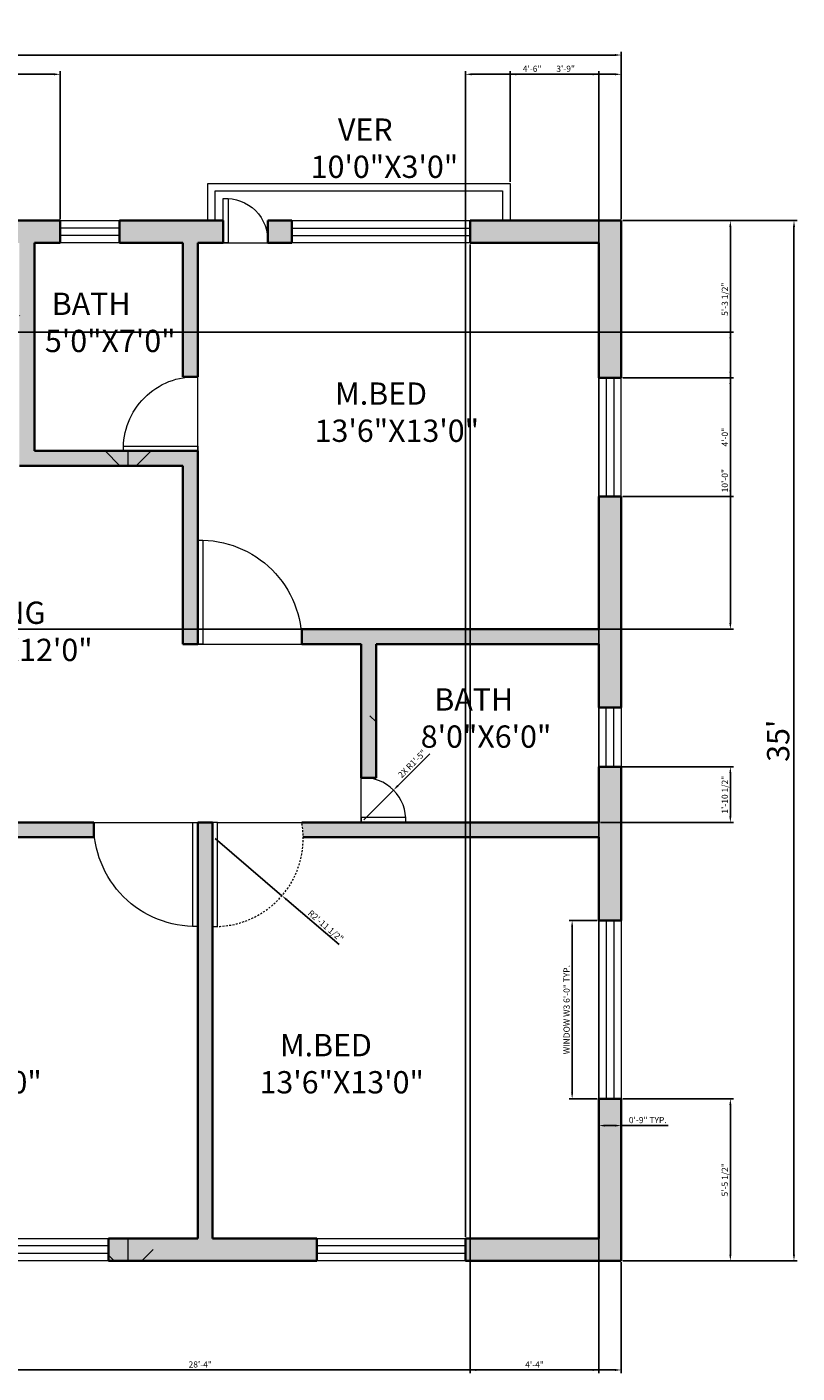
# Model space of a CAD drawing. Units: inches. Extents: x 1851 to 3979, y 3948 to 8145.
# Tile 4 of 4: x 2438 to 2749, y 3948 to 4491. Entities that reach past the tile are written whole.
import ezdxf

# ---------------------------------------------------------------- set-up
doc = ezdxf.new("R2010")
doc.units = ezdxf.units.IN
doc.linetypes.add('JIS_02_0.7', pattern=[1.35, 0.75, -0.6])
for name, color, linetype, lineweight in [('A-ANNO-DIMS', 2, 'Continuous', 18), ('A-GLAZ', 140, 'Continuous', 18), ('A-WALL', 7, 'Continuous', 35)]:
    doc.layers.add(name, color=color, linetype=linetype, lineweight=lineweight)
for name, color, linetype, lineweight, true_color in [('A-AREA-IDEN', 9, 'Continuous', 18, 0xc7c8ca), ('A-DOOR', 52, 'Continuous', 18, 0xc8c92d), ('A-DOOR-SWNG', 52, 'JIS_02_0.7', 13, 0xc8c92d), ('A-FLOR-RAIL', 52, 'Continuous', 18, 0xc8c92d), ('A-WALL-PATT', 159, 'Continuous', 13, 0x22346e)]:
    doc.layers.add(name, color=color, linetype=linetype, lineweight=lineweight, true_color=true_color)
doc.styles.get("Standard").update_dxf_attribs({"font": 'arial.ttf'})
doc.dimstyles.new('ISO-25', dxfattribs={"dimtxt": 2.5, "dimasz": 2.5, "dimexe": 1.25, "dimexo": 0.625, "dimtad": 1, "dimlunit": 3, "dimtxsty": 'Standard', "dimcen": 2.5, "dimadec": 0, "dimazin": 0, "dimtfac": 1, "dimtmove": 0, "dimatfit": 3, "dimfxl": 1, "dimarcsym": 0})

# ---------------------------------------------------------------- blocks, each defined once
blk = doc.blocks.new('*D1')
at = {"layer": 'A-ANNO-DIMS', "color": 0, "lineweight": -2, "transparency": 16777216}
for p, q in [((1898.74, 4438.02), (1898.74, 4480.98)), ((1901.24, 4479.73), (2675.24, 4479.73)), ((2677.74, 4438.02), (2677.74, 4480.98))]:
    blk.add_line(p, q, dxfattribs=at)
at = {"layer": 'A-ANNO-DIMS', "color": 0, "transparency": 16777216}
for points in [[(1901.24, 4480.15), (1901.24, 4479.31), (1898.74, 4479.73)], [(2675.24, 4480.15), (2675.24, 4479.31), (2677.74, 4479.73)]]:
    blk.add_solid(points, dxfattribs=at)
at = {"layer": 'Defpoints', "color": 0, "transparency": 16777216}
for p in [(2677.74, 4479.73), (1898.74, 4437.39), (2677.74, 4437.39)]:
    blk.add_point(p, dxfattribs=at)
at = {"layer": 'A-ANNO-DIMS', "color": 0, "transparency": 16777216, "insert": (2288.24, 4484.95), "char_height": 9, "attachment_point": 5}
blk.add_mtext('64\'-11"', dxfattribs=at)
blk = doc.blocks.new('*D2')
at = {"layer": 'A-ANNO-DIMS', "color": 0, "lineweight": -2, "transparency": 16777216}
for p, q in [((2712.32, 4412.85), (2748.78, 4412.85)), ((2747.53, 4410.35), (2747.53, 3995.35)), ((2699.58, 3992.85), (2748.78, 3992.85))]:
    blk.add_line(p, q, dxfattribs=at)
at = {"layer": 'A-ANNO-DIMS', "color": 0, "transparency": 16777216}
for points in [[(2747.12, 4410.35), (2747.95, 4410.35), (2747.53, 4412.85)], [(2747.12, 3995.35), (2747.95, 3995.35), (2747.53, 3992.85)]]:
    blk.add_solid(points, dxfattribs=at)
at = {"layer": 'Defpoints', "color": 0, "transparency": 16777216}
for p in [(2711.7, 4412.85), (2698.96, 3992.85), (2747.53, 3992.85)]:
    blk.add_point(p, dxfattribs=at)
at = {"layer": 'A-ANNO-DIMS', "color": 0, "transparency": 16777216, "insert": (2742.31, 4202.85), "char_height": 9, "attachment_point": 5, "rotation": 90}
blk.add_mtext("35'", dxfattribs=at)
blk = doc.blocks.new('DOOR-SINGLE-42IN')
for p, q in [((42, 42), (40, 42)), ((40, 42), (40, 0)), ((42, 0), (42, 42)), ((40, 0), (42, 0))]:
    blk.add_line(p, q)
blk.add_arc((41, 1), 41.01, 88.6028, 181.3972)
blk = doc.blocks.new('DOOR-SINGLE-30IN')
for p, q in [((30, 2), (0, 2)), ((0, 2), (0, 0)), ((0, 0), (30, 0)), ((30, 0), (30, 2))]:
    blk.add_line(p, q)
blk.add_arc((1, 1), 29.02, 358.0251, 91.9749)
blk = doc.blocks.new('DOOR-SINGLE-18IN')
for p, q in [((18, 18), (16, 18)), ((16, 18), (16, 0)), ((18, 0), (18, 18)), ((16, 0), (18, 0))]:
    blk.add_line(p, q)
blk.add_arc((17, 1), 17.03, 86.6335, 183.3665)
blk = doc.blocks.new('WINDOW-60IN')
for p, q in [((0, 9), (60, 9)), ((0, 0), (0, 9)), ((0, 6), (60, 6)), ((60, 9), (60, 0)), ((0, 3), (60, 3)), ((60, 0), (0, 0))]:
    blk.add_line(p, q)
blk = doc.blocks.new('WINDOW-24IN')
for p, q in [((0, 0), (0, 9)), ((0, 9), (24, 9)), ((0, 6), (24, 6)), ((24, 9), (24, 0)), ((0, 3), (24, 3)), ((24, 0), (0, 0))]:
    blk.add_line(p, q)
blk = doc.blocks.new('WINDOW-72IN')
for p, q in [((0, 9), (72, 9)), ((0, 0), (0, 9)), ((0, 6), (72, 6)), ((72, 9), (72, 0)), ((0, 3), (72, 3)), ((72, 0), (0, 0))]:
    blk.add_line(p, q)
blk = doc.blocks.new('*D14')
at = {"layer": 'A-ANNO-DIMS', "color": 0, "lineweight": -2, "transparency": 16777216}
for p, q in [((2668.11, 4130.25), (2656.69, 4130.25)), ((2657.94, 4127.75), (2657.94, 4060.75)), ((2668.11, 4058.25), (2656.69, 4058.25))]:
    blk.add_line(p, q, dxfattribs=at)
at = {"layer": 'A-ANNO-DIMS', "color": 0, "transparency": 16777216}
for points in [[(2657.52, 4127.75), (2658.35, 4127.75), (2657.94, 4130.25)], [(2657.52, 4060.75), (2658.35, 4060.75), (2657.94, 4058.25)]]:
    blk.add_solid(points, dxfattribs=at)
at = {"layer": 'Defpoints', "color": 0, "transparency": 16777216}
for p in [(2668.74, 4130.25), (2657.94, 4058.25), (2668.74, 4058.25)]:
    blk.add_point(p, dxfattribs=at)
at = {"layer": 'A-ANNO-DIMS', "color": 0, "transparency": 16777216, "insert": (2656.02, 4094.25), "char_height": 2.5, "attachment_point": 5, "rotation": 90}
blk.add_mtext('WINDOW W3 6\'-0" TYP.', dxfattribs=at)
blk = doc.blocks.new('*D15')
at = {"layer": 'A-ANNO-DIMS', "color": 0, "lineweight": -2, "transparency": 16777216}
for p, q in [((2668.74, 4057.63), (2668.74, 4046.2)), ((2677.74, 4057.63), (2677.74, 4046.2)), ((2671.24, 4047.45), (2675.24, 4047.45)), ((2677.74, 4047.45), (2696.72, 4047.45))]:
    blk.add_line(p, q, dxfattribs=at)
at = {"layer": 'A-ANNO-DIMS', "color": 0, "transparency": 16777216}
for points in [[(2671.24, 4047.87), (2671.24, 4047.03), (2668.74, 4047.45)], [(2675.24, 4047.87), (2675.24, 4047.03), (2677.74, 4047.45)]]:
    blk.add_solid(points, dxfattribs=at)
at = {"layer": 'Defpoints', "color": 0, "transparency": 16777216}
for p in [(2668.74, 4058.25), (2677.74, 4058.25), (2677.74, 4047.45)]:
    blk.add_point(p, dxfattribs=at)
at = {"layer": 'A-ANNO-DIMS', "color": 0, "transparency": 16777216, "insert": (2688.48, 4049.35), "char_height": 2.5, "attachment_point": 5}
blk.add_mtext('0\'-9" TYP.', dxfattribs=at)
blk = doc.blocks.new('*D26')
at = {"layer": 'A-ANNO-DIMS', "color": 0, "lineweight": -2, "transparency": 16777216}
for p, q in [((2337.74, 3992.23), (2337.74, 3947.5)), ((2677.74, 3992.23), (2677.74, 3947.5)), ((2340.24, 3948.75), (2675.24, 3948.75))]:
    blk.add_line(p, q, dxfattribs=at)
at = {"layer": 'A-ANNO-DIMS', "color": 0, "transparency": 16777216}
for points in [[(2340.24, 3949.17), (2340.24, 3948.34), (2337.74, 3948.75)], [(2675.24, 3949.17), (2675.24, 3948.34), (2677.74, 3948.75)]]:
    blk.add_solid(points, dxfattribs=at)
at = {"layer": 'Defpoints', "color": 0, "transparency": 16777216}
for p in [(2337.74, 3992.85), (2677.74, 3992.85), (2677.74, 3948.75)]:
    blk.add_point(p, dxfattribs=at)
at = {"layer": 'A-ANNO-DIMS', "color": 0, "transparency": 16777216, "insert": (2507.74, 3950.66), "char_height": 2.5, "attachment_point": 5}
blk.add_mtext('28\'-4"', dxfattribs=at)
blk = doc.blocks.new('*D30')
at = {"layer": 'A-ANNO-DIMS', "color": 0, "lineweight": -2, "transparency": 16777216}
for p, q in [((2614.83, 4002.48), (2614.83, 4473.2)), ((2617.33, 4471.95), (2666.24, 4471.95)), ((2668.74, 4002.48), (2668.74, 4473.2))]:
    blk.add_line(p, q, dxfattribs=at)
at = {"layer": 'A-ANNO-DIMS', "color": 0, "transparency": 16777216}
for points in [[(2617.33, 4472.37), (2617.33, 4471.54), (2614.83, 4471.95)], [(2666.24, 4472.37), (2666.24, 4471.54), (2668.74, 4471.95)]]:
    blk.add_solid(points, dxfattribs=at)
at = {"layer": 'Defpoints', "color": 0, "transparency": 16777216}
for p in [(2668.74, 4471.95), (2614.83, 4001.85), (2668.74, 4001.85)]:
    blk.add_point(p, dxfattribs=at)
at = {"layer": 'A-ANNO-DIMS', "color": 0, "transparency": 16777216, "insert": (2641.78, 4473.86), "char_height": 2.5, "attachment_point": 5}
blk.add_mtext('4\'-6"', dxfattribs=at)
blk = doc.blocks.new('*D32')
at = {"layer": 'A-ANNO-DIMS', "color": 0, "lineweight": -2, "transparency": 16777216}
for p, q in [((2632.88, 4428.48), (2632.88, 4473.2)), ((2635.38, 4471.95), (2675.24, 4471.95)), ((2677.74, 4413.48), (2677.74, 4473.2))]:
    blk.add_line(p, q, dxfattribs=at)
at = {"layer": 'A-ANNO-DIMS', "color": 0, "transparency": 16777216}
for points in [[(2635.38, 4472.37), (2635.38, 4471.54), (2632.88, 4471.95)], [(2675.24, 4472.37), (2675.24, 4471.54), (2677.74, 4471.95)]]:
    blk.add_solid(points, dxfattribs=at)
at = {"layer": 'Defpoints', "color": 0, "transparency": 16777216}
for p in [(2677.74, 4471.95), (2632.88, 4427.85), (2677.74, 4412.85)]:
    blk.add_point(p, dxfattribs=at)
at = {"layer": 'A-ANNO-DIMS', "color": 0, "transparency": 16777216, "insert": (2655.31, 4473.86), "char_height": 2.5, "attachment_point": 5}
blk.add_mtext('3\'-9"', dxfattribs=at)
blk = doc.blocks.new('*D33')
at = {"layer": 'A-ANNO-DIMS', "color": 0, "lineweight": -2, "transparency": 16777216}
for p, q in [((2245.36, 4367.85), (2723.09, 4367.85)), ((2721.84, 4250.35), (2721.84, 4365.35)), ((2245.36, 4247.85), (2723.09, 4247.85))]:
    blk.add_line(p, q, dxfattribs=at)
at = {"layer": 'A-ANNO-DIMS', "color": 0, "transparency": 16777216}
for points in [[(2721.42, 4365.35), (2722.25, 4365.35), (2721.84, 4367.85)], [(2721.42, 4250.35), (2722.25, 4250.35), (2721.84, 4247.85)]]:
    blk.add_solid(points, dxfattribs=at)
at = {"layer": 'Defpoints', "color": 0, "transparency": 16777216}
for p in [(2244.74, 4367.85), (2721.84, 4367.85), (2244.74, 4247.85)]:
    blk.add_point(p, dxfattribs=at)
at = {"layer": 'A-ANNO-DIMS', "color": 0, "transparency": 16777216, "insert": (2719.93, 4307.85), "char_height": 2.5, "attachment_point": 5, "rotation": 90}
blk.add_mtext('10\'-0"', dxfattribs=at)
blk = doc.blocks.new('*D40')
at = {"layer": 'A-ANNO-DIMS', "color": 0, "lineweight": -2, "transparency": 16777216}
for p, q in [((2678.36, 4058.25), (2723.09, 4058.25)), ((2721.84, 3995.35), (2721.84, 4055.75)), ((2678.36, 3992.85), (2723.09, 3992.85))]:
    blk.add_line(p, q, dxfattribs=at)
at = {"layer": 'A-ANNO-DIMS', "color": 0, "transparency": 16777216}
for points in [[(2721.42, 4055.75), (2722.25, 4055.75), (2721.84, 4058.25)], [(2721.42, 3995.35), (2722.25, 3995.35), (2721.84, 3992.85)]]:
    blk.add_solid(points, dxfattribs=at)
at = {"layer": 'Defpoints', "color": 0, "transparency": 16777216}
for p in [(2677.74, 4058.25), (2721.84, 4058.25), (2677.74, 3992.85)]:
    blk.add_point(p, dxfattribs=at)
at = {"layer": 'A-ANNO-DIMS', "color": 0, "transparency": 16777216, "insert": (2719.92, 4025.55), "char_height": 2.5, "attachment_point": 5, "rotation": 90}
blk.add_mtext('5\'-5 1/2"', dxfattribs=at)
blk = doc.blocks.new('*D41')
at = {"layer": 'A-ANNO-DIMS', "color": 0, "lineweight": -2, "transparency": 16777216}
for p, q in [((2669.36, 4192.25), (2723.09, 4192.25)), ((2721.84, 4172.35), (2721.84, 4189.75)), ((2669.36, 4169.85), (2723.09, 4169.85))]:
    blk.add_line(p, q, dxfattribs=at)
at = {"layer": 'A-ANNO-DIMS', "color": 0, "transparency": 16777216}
for points in [[(2721.42, 4189.75), (2722.25, 4189.75), (2721.84, 4192.25)], [(2721.42, 4172.35), (2722.25, 4172.35), (2721.84, 4169.85)]]:
    blk.add_solid(points, dxfattribs=at)
at = {"layer": 'Defpoints', "color": 0, "transparency": 16777216}
for p in [(2668.74, 4192.25), (2721.84, 4192.25), (2668.74, 4169.85)]:
    blk.add_point(p, dxfattribs=at)
at = {"layer": 'A-ANNO-DIMS', "color": 0, "transparency": 16777216, "insert": (2719.92, 4181.05), "char_height": 2.5, "attachment_point": 5, "rotation": 90}
blk.add_mtext('1\'-10 1/2"', dxfattribs=at)
blk = doc.blocks.new('*D42')
at = {"layer": 'A-ANNO-DIMS', "color": 0, "lineweight": -2, "transparency": 16777216}
for p, q in [((2678.36, 4349.41), (2723.09, 4349.41)), ((2721.84, 4303.91), (2721.84, 4346.91)), ((2678.36, 4301.41), (2723.09, 4301.41))]:
    blk.add_line(p, q, dxfattribs=at)
at = {"layer": 'A-ANNO-DIMS', "color": 0, "transparency": 16777216}
for points in [[(2721.42, 4346.91), (2722.25, 4346.91), (2721.84, 4349.41)], [(2721.42, 4303.91), (2722.25, 4303.91), (2721.84, 4301.41)]]:
    blk.add_solid(points, dxfattribs=at)
at = {"layer": 'Defpoints', "color": 0, "transparency": 16777216}
for p in [(2677.74, 4349.41), (2721.84, 4349.41), (2677.74, 4301.41)]:
    blk.add_point(p, dxfattribs=at)
at = {"layer": 'A-ANNO-DIMS', "color": 0, "transparency": 16777216, "insert": (2719.93, 4325.41), "char_height": 2.5, "attachment_point": 5, "rotation": 90}
blk.add_mtext('4\'-0"', dxfattribs=at)
blk = doc.blocks.new('*D43')
at = {"layer": 'A-ANNO-DIMS', "color": 0, "lineweight": -2, "transparency": 16777216}
for p, q in [((2678.36, 4412.85), (2723.09, 4412.85)), ((2721.84, 4351.91), (2721.84, 4410.35)), ((2678.36, 4349.41), (2723.09, 4349.41))]:
    blk.add_line(p, q, dxfattribs=at)
at = {"layer": 'A-ANNO-DIMS', "color": 0, "transparency": 16777216}
for points in [[(2721.42, 4410.35), (2722.25, 4410.35), (2721.84, 4412.85)], [(2721.42, 4351.91), (2722.25, 4351.91), (2721.84, 4349.41)]]:
    blk.add_solid(points, dxfattribs=at)
at = {"layer": 'Defpoints', "color": 0, "transparency": 16777216}
for p in [(2677.74, 4412.85), (2721.84, 4412.85), (2677.74, 4349.41)]:
    blk.add_point(p, dxfattribs=at)
at = {"layer": 'A-ANNO-DIMS', "color": 0, "transparency": 16777216, "insert": (2719.92, 4381.13), "char_height": 2.5, "attachment_point": 5, "rotation": 90}
blk.add_mtext('5\'-3 1/2"', dxfattribs=at)
blk = doc.blocks.new('*D47')
at = {"layer": 'A-ANNO-DIMS', "color": 0, "lineweight": -2, "transparency": 16777216}
for p, q in [((2616.74, 4403.23), (2616.74, 3947.5)), ((2668.74, 4403.23), (2668.74, 3947.5)), ((2619.24, 3948.75), (2666.24, 3948.75))]:
    blk.add_line(p, q, dxfattribs=at)
at = {"layer": 'A-ANNO-DIMS', "color": 0, "transparency": 16777216}
for points in [[(2619.24, 3949.17), (2619.24, 3948.34), (2616.74, 3948.75)], [(2666.24, 3949.17), (2666.24, 3948.34), (2668.74, 3948.75)]]:
    blk.add_solid(points, dxfattribs=at)
at = {"layer": 'Defpoints', "color": 0, "transparency": 16777216}
for p in [(2616.74, 4403.85), (2668.74, 4403.85), (2668.74, 3948.75)]:
    blk.add_point(p, dxfattribs=at)
at = {"layer": 'A-ANNO-DIMS', "color": 0, "transparency": 16777216, "insert": (2642.74, 3950.63), "char_height": 2.5, "attachment_point": 5}
blk.add_mtext('4\'-4"', dxfattribs=at)
blk = doc.blocks.new('*D52')
at = {"layer": 'A-ANNO-DIMS', "color": 0, "lineweight": -2, "transparency": 16777216}
for p, q in [((2401.88, 4413.48), (2401.88, 4473.2)), ((2404.38, 4471.95), (2448.67, 4471.95)), ((2451.17, 4413.48), (2451.17, 4473.2))]:
    blk.add_line(p, q, dxfattribs=at)
at = {"layer": 'A-ANNO-DIMS', "color": 0, "transparency": 16777216}
for points in [[(2404.38, 4472.37), (2404.38, 4471.54), (2401.88, 4471.95)], [(2448.67, 4472.37), (2448.67, 4471.54), (2451.17, 4471.95)]]:
    blk.add_solid(points, dxfattribs=at)
at = {"layer": 'Defpoints', "color": 0, "transparency": 16777216}
for p in [(2451.17, 4471.95), (2401.88, 4412.85), (2451.17, 4412.85)]:
    blk.add_point(p, dxfattribs=at)
at = {"layer": 'A-ANNO-DIMS', "color": 0, "transparency": 16777216, "insert": (2426.53, 4473.87), "char_height": 2.5, "attachment_point": 5}
blk.add_mtext('4\'-1 1/2"', dxfattribs=at)
blk = doc.blocks.new('*D54')
at = {"layer": 'A-ANNO-DIMS', "color": 0, "lineweight": -2, "transparency": 16777216}
for p, q in [((2513.74, 4163.43), (2540.75, 4140.27)), ((2563.82, 4120.5), (2542.65, 4138.64))]:
    blk.add_line(p, q, dxfattribs=at)
at = {"layer": 'A-ANNO-DIMS', "color": 0, "transparency": 16777216}
blk.add_solid([(2542.92, 4138.96), (2542.38, 4138.32), (2540.75, 4140.27)], dxfattribs=at)
at = {"layer": 'Defpoints', "color": 0, "transparency": 16777216}
for p in [(2513.74, 4163.43), (2540.75, 4140.27)]:
    blk.add_point(p, dxfattribs=at)
at = {"layer": 'A-ANNO-DIMS', "color": 0, "transparency": 16777216, "insert": (2558.21, 4127.83), "char_height": 2.5, "attachment_point": 5, "rotation": 319.3996}
blk.add_mtext('R2\'-11 1/2"', dxfattribs=at)
blk = doc.blocks.new('*D56')
at = {"layer": 'A-ANNO-DIMS', "color": 0, "lineweight": -2, "transparency": 16777216}
for p, q in [((2600.42, 4197.54), (2587.55, 4184.66)), ((2573.74, 4170.85), (2585.78, 4182.9))]:
    blk.add_line(p, q, dxfattribs=at)
at = {"layer": 'A-ANNO-DIMS', "color": 0, "transparency": 16777216}
blk.add_solid([(2587.25, 4184.96), (2587.84, 4184.37), (2585.78, 4182.9)], dxfattribs=at)
at = {"layer": 'Defpoints', "color": 0, "transparency": 16777216}
for p in [(2585.78, 4182.9), (2573.74, 4170.85)]:
    blk.add_point(p, dxfattribs=at)
at = {"layer": 'A-ANNO-DIMS', "color": 0, "transparency": 16777216, "insert": (2593.52, 4193.33), "char_height": 2.5, "attachment_point": 5, "rotation": 45.0002}
blk.add_mtext('2X R1\'-5"', dxfattribs=at)

msp = doc.modelspace()

# ---------------------------------------------------------------- hatches: boundary and pattern name
at = {"layer": 'A-WALL-PATT'}
h = msp.add_hatch(dxfattribs=at)
h.set_pattern_fill('GRASS', color=256, scale=3)
h.paths.add_polyline_path([(1942.655, 4412.855), (1898.736, 4412.855), (1898.736, 4348.625), (1907.736, 4348.625), (1907.736, 4403.855), (1942.655, 4403.855)])
h.paths.add_polyline_path([(2027.97, 4412.855), (2002.655, 4412.855), (2002.655, 4403.855), (2027.97, 4403.855, -0.0293864), (2027.97, 4405.855)])
h.paths.add_polyline_path([(2088.59, 4412.855), (2045.97, 4412.855), (2045.97, 4403.855), (2069.736, 4403.855), (2069.736, 4349.855, -0.0172363), (2071.736, 4349.855), (2075.736, 4349.855), (2075.736, 4403.855), (2088.59, 4403.855)])
h.paths.add_polyline_path([(2158.724, 4412.855), (2112.59, 4412.855), (2112.59, 4403.855), (2135.736, 4403.855), (2135.736, 4319.855), (2069.736, 4319.855), (2069.736, 4241.855), (2075.736, 4241.855), (2075.736, 4313.855), (2141.736, 4313.855), (2141.736, 4403.855), (2158.724, 4403.855)])
h.paths.add_polyline_path([(2244.736, 4403.855), (2256.687, 4403.855), (2256.687, 4412.855), (2218.724, 4412.855), (2218.724, 4403.855), (2238.736, 4403.855), (2238.736, 4319.855), (2171.736, 4319.855), (2171.736, 4315.855, -0.0172363), (2171.736, 4313.855), (2238.736, 4313.855), (2238.736, 4211.855), (2242.736, 4211.855, -0.0121933), (2244.736, 4211.855)])
h.paths.add_polyline_path([(2356.912, 4412.855), (2353.884, 4412.855), (2312.372, 4412.855), (2312.372, 4403.855), (2331.736, 4403.855), (2331.736, 4211.855, -0.0121933), (2333.736, 4211.855), (2337.736, 4211.855), (2337.736, 4313.855), (2404.736, 4313.855, -0.0172363), (2404.736, 4315.855), (2404.736, 4319.855), (2337.736, 4319.855), (2337.736, 4403.855), (2353.884, 4403.855), (2356.912, 4403.855)])
h.paths.add_polyline_path([(2440.736, 4403.855), (2451.168, 4403.855), (2451.168, 4412.855), (2401.884, 4412.855), (2401.884, 4403.855), (2434.736, 4403.855), (2434.736, 4313.855), (2500.736, 4313.855), (2500.736, 4241.855), (2506.736, 4241.855), (2506.736, 4283.855), (2506.736, 4319.855), (2476.736, 4319.855), (2440.736, 4319.855)])
h.paths.add_polyline_path([(2506.736, 4403.855), (2516.983, 4403.855), (2516.983, 4412.855), (2475.168, 4412.855), (2475.168, 4403.855), (2500.736, 4403.855), (2500.736, 4349.855), (2504.736, 4349.855, -0.0172363), (2506.736, 4349.855)])
h.paths.add_polyline_path([(2544.739, 4412.855), (2534.983, 4412.855), (2534.983, 4405.855, -0.0293864), (2534.983, 4403.855), (2544.739, 4403.855)])
h.paths.add_polyline_path([(2677.736, 4412.855), (2618.736, 4412.855), (2616.739, 4412.855), (2616.739, 4403.855), (2668.736, 4403.855), (2668.736, 4349.414), (2677.736, 4349.414), (2677.736, 4403.855)])
h.paths.add_polyline_path([(2677.736, 4301.414), (2668.736, 4301.414), (2668.736, 4247.855), (2548.736, 4247.855), (2548.736, 4243.855, -0.0121933), (2548.736, 4241.855), (2572.736, 4241.855), (2572.736, 4187.855, -0.0293864), (2574.736, 4187.855), (2578.736, 4187.855), (2578.736, 4241.855), (2668.736, 4241.855), (2668.736, 4216.247), (2677.736, 4216.247)])
h.paths.add_polyline_path([(2677.736, 4192.247), (2668.736, 4192.247), (2668.736, 4169.855), (2572.736, 4169.855), (2548.736, 4169.855, -0.0424267), (2549.319, 4163.855), (2572.736, 4163.855), (2668.736, 4163.855), (2668.736, 4130.251), (2677.736, 4130.251)])
h.paths.add_polyline_path([(2677.736, 4001.855), (2677.736, 4058.251), (2668.736, 4058.251), (2668.736, 4001.855), (2614.828, 4001.855), (2614.828, 3992.855), (2618.736, 3992.855), (2677.736, 3992.855)])
h.paths.add_polyline_path([(2554.828, 4001.855), (2512.736, 4001.855), (2512.736, 4163.855), (2512.736, 4169.855), (2506.736, 4169.855), (2506.736, 4127.855), (2506.736, 4001.855), (2470.736, 4001.855), (2470.736, 3992.855), (2554.828, 3992.855)])
h.paths.add_polyline_path([(2410.736, 4001.855), (2337.736, 4001.855), (2337.736, 3992.855), (2410.736, 3992.855)])
h.paths.add_polyline_path([(2337.736, 4169.855), (2331.736, 4169.855), (2331.736, 4075.855), (2337.736, 4075.855)])
h.paths.add_polyline_path([(2464.736, 4167.855, -0.0121933), (2464.736, 4169.855), (2337.736, 4169.855), (2337.736, 4163.855), (2464.736, 4163.855)])
h.paths.add_polyline_path([(2244.736, 4169.855), (2202.736, 4169.855), (2117.736, 4169.855, -0.0121933), (2117.736, 4167.855), (2117.736, 4163.855), (2238.736, 4163.855), (2238.736, 4075.855), (2244.736, 4075.855)])
h.paths.add_polyline_path([(2325.736, 4001.855), (2250.736, 4001.855), (2250.736, 3992.855), (2325.736, 3992.855)])
h.paths.add_polyline_path([(2238.736, 4001.855), (2175.511, 4001.855), (2175.511, 3992.855), (2238.736, 3992.855)])
h.paths.add_polyline_path([(2115.511, 4001.855), (2075.736, 4001.855), (2075.736, 4169.855), (2069.736, 4169.855), (2069.736, 4127.855), (2069.736, 4001.855), (2009.539, 4001.855), (2009.539, 3992.855), (2115.511, 3992.855)])
h.paths.add_polyline_path([(1949.539, 4001.855), (1907.736, 4001.855), (1907.736, 4049.088), (1898.736, 4049.088), (1898.736, 3992.855), (1949.539, 3992.855)])
h.paths.add_polyline_path([(1907.736, 4163.855), (2027.736, 4163.855), (2027.736, 4167.855, -0.0121933), (2027.736, 4169.855), (1907.736, 4169.855), (1907.736, 4195.575), (1898.736, 4195.575), (1898.736, 4109.088), (1907.736, 4109.088)])
h.paths.add_polyline_path([(2027.736, 4247.855), (1907.736, 4247.855), (1907.736, 4288.625), (1898.736, 4288.625), (1898.736, 4219.575), (1907.736, 4219.575), (1907.736, 4241.855), (2003.736, 4241.855), (2003.736, 4219.575), (2003.736, 4199.855), (2007.736, 4199.855, -0.0172363), (2009.736, 4199.855), (2009.736, 4241.855), (2027.736, 4241.855, -0.0121933), (2027.736, 4243.855)])
h = msp.add_hatch(color=256, dxfattribs=at)
h.dxf.hatch_style = 1
h.paths.add_polyline_path([(1907.736, 4163.855), (2027.736, 4163.855), (2027.736, 4167.855, -0.0121933), (2027.736, 4169.855), (1907.736, 4169.855), (1907.736, 4195.575), (1898.736, 4195.575), (1898.736, 4109.088), (1907.736, 4109.088)])
h.paths.add_polyline_path([(1907.736, 4049.088), (1898.736, 4049.088), (1898.736, 3992.855), (1949.539, 3992.855), (1949.539, 4001.855), (1907.736, 4001.855)])
h.paths.add_polyline_path([(2115.511, 4001.855), (2075.736, 4001.855), (2075.736, 4169.855), (2069.736, 4169.855), (2069.736, 4127.855), (2069.736, 4001.855), (2009.539, 4001.855), (2009.539, 3992.855), (2115.511, 3992.855)])
h.paths.add_polyline_path([(2238.736, 4001.855), (2175.511, 4001.855), (2175.511, 3992.855), (2238.736, 3992.855)])
h.paths.add_polyline_path([(2325.736, 4001.855), (2250.736, 4001.855), (2250.736, 3992.855), (2325.736, 3992.855)])
h.paths.add_polyline_path([(2410.736, 4001.855), (2337.736, 4001.855), (2337.736, 3992.855), (2410.736, 3992.855)])
h.paths.add_polyline_path([(2554.828, 4001.855), (2512.736, 4001.855), (2512.736, 4163.855), (2512.736, 4169.855), (2506.736, 4169.855), (2506.736, 4127.855), (2506.736, 4001.855), (2470.736, 4001.855), (2470.736, 3992.855), (2554.828, 3992.855)])
h.paths.add_polyline_path([(2677.736, 4001.855), (2677.736, 4058.251), (2668.736, 4058.251), (2668.736, 4001.855), (2614.828, 4001.855), (2614.828, 3992.855), (2618.736, 3992.855), (2677.736, 3992.855)])
h.paths.add_polyline_path([(2244.736, 4169.855), (2202.736, 4169.855), (2117.736, 4169.855, -0.0121933), (2117.736, 4167.855), (2117.736, 4163.855), (2238.736, 4163.855), (2238.736, 4075.855), (2244.736, 4075.855)])
h.paths.add_polyline_path([(2337.736, 4169.855), (2331.736, 4169.855), (2331.736, 4075.855), (2337.736, 4075.855)])
h.paths.add_polyline_path([(2337.736, 4063.855), (2331.736, 4063.855), (2331.736, 4004.855), (2337.736, 4004.855)])
h.paths.add_polyline_path([(2244.736, 4063.855), (2238.736, 4063.855), (2238.736, 4004.855), (2244.736, 4004.855)])
h.paths.add_polyline_path([(2464.736, 4167.855, -0.0121933), (2464.736, 4169.855), (2337.736, 4169.855), (2337.736, 4163.855), (2464.736, 4163.855)])
h.paths.add_polyline_path([(2337.736, 4313.855), (2404.736, 4313.855, -0.0172363), (2404.736, 4315.855), (2404.736, 4319.855), (2337.736, 4319.855), (2337.736, 4403.855), (2353.884, 4403.855), (2356.912, 4403.855), (2356.912, 4412.855), (2353.884, 4412.855), (2312.372, 4412.855), (2312.372, 4403.855), (2331.736, 4403.855), (2331.736, 4211.855, -0.0121933), (2333.736, 4211.855), (2337.736, 4211.855)])
h.paths.add_polyline_path([(2244.736, 4403.855), (2256.687, 4403.855), (2256.687, 4412.855), (2218.724, 4412.855), (2218.724, 4403.855), (2238.736, 4403.855), (2238.736, 4319.855), (2171.736, 4319.855), (2171.736, 4315.855, -0.0172363), (2171.736, 4313.855), (2238.736, 4313.855), (2238.736, 4211.855), (2242.736, 4211.855, -0.0121933), (2244.736, 4211.855)])
h.paths.add_polyline_path([(2506.736, 4283.855), (2506.736, 4319.855), (2476.736, 4319.855), (2440.736, 4319.855), (2440.736, 4403.855), (2451.168, 4403.855), (2451.168, 4412.855), (2401.884, 4412.855), (2401.884, 4403.855), (2434.736, 4403.855), (2434.736, 4313.855), (2500.736, 4313.855), (2500.736, 4241.855), (2506.736, 4241.855)])
h.paths.add_polyline_path([(2578.736, 4241.855), (2668.736, 4241.855), (2668.736, 4216.247), (2677.736, 4216.247), (2677.736, 4301.414), (2668.736, 4301.414), (2668.736, 4247.855), (2548.736, 4247.855), (2548.736, 4243.855, -0.0121933), (2548.736, 4241.855), (2572.736, 4241.855), (2572.736, 4187.855, -0.0293864), (2574.736, 4187.855), (2578.736, 4187.855)])
h.paths.add_polyline_path([(2677.736, 4192.247), (2668.736, 4192.247), (2668.736, 4169.855), (2572.736, 4169.855), (2548.736, 4169.855, -0.0424267), (2549.319, 4163.855), (2572.736, 4163.855), (2668.736, 4163.855), (2668.736, 4130.251), (2677.736, 4130.251)])
h.paths.add_polyline_path([(2506.736, 4403.855), (2516.983, 4403.855), (2516.983, 4412.855), (2475.168, 4412.855), (2475.168, 4403.855), (2500.736, 4403.855), (2500.736, 4349.855), (2504.736, 4349.855, -0.0172363), (2506.736, 4349.855)])
h.paths.add_polyline_path([(2677.736, 4412.855), (2618.736, 4412.855), (2616.739, 4412.855), (2616.739, 4403.855), (2668.736, 4403.855), (2668.736, 4349.414), (2677.736, 4349.414), (2677.736, 4403.855)])
h.paths.add_polyline_path([(2544.739, 4412.855), (2534.983, 4412.855), (2534.983, 4405.855, -0.0293864), (2534.983, 4403.855), (2544.739, 4403.855)])
h.paths.add_polyline_path([(2141.736, 4403.855), (2158.724, 4403.855), (2158.724, 4412.855), (2112.59, 4412.855), (2112.59, 4403.855), (2135.736, 4403.855), (2135.736, 4319.855), (2069.736, 4319.855), (2069.736, 4241.855), (2075.736, 4241.855), (2075.736, 4313.855), (2141.736, 4313.855), (2141.736, 4343.855)])
h.paths.add_polyline_path([(2075.736, 4403.855), (2088.59, 4403.855), (2088.59, 4412.855), (2045.97, 4412.855), (2045.97, 4403.855), (2069.736, 4403.855), (2069.736, 4349.855, -0.0172363), (2071.736, 4349.855), (2075.736, 4349.855)])
h.paths.add_polyline_path([(2027.97, 4412.855), (2002.655, 4412.855), (2002.655, 4403.855), (2027.97, 4403.855, -0.0293864), (2027.97, 4405.855)])
h.paths.add_polyline_path([(1942.655, 4412.855), (1898.736, 4412.855), (1898.736, 4348.625), (1907.736, 4348.625), (1907.736, 4403.855), (1942.655, 4403.855)])
h.paths.add_polyline_path([(2027.736, 4247.855), (1907.736, 4247.855), (1907.736, 4288.625), (1898.736, 4288.625), (1898.736, 4219.575), (1907.736, 4219.575), (1907.736, 4241.855), (2003.736, 4241.855), (2003.736, 4219.575), (2003.736, 4199.855), (2007.736, 4199.855, -0.0172363), (2009.736, 4199.855), (2009.736, 4241.855), (2027.736, 4241.855, -0.0121933), (2027.736, 4243.855)])

# ---------------------------------------------------------------- linework, layer by layer
at = {"layer": 'A-DOOR'}
for p, q in [((2516.983, 4403.855), (2534.983, 4403.855)), ((2506.736, 4319.855), (2506.736, 4349.855)), ((2506.736, 4241.855), (2548.736, 4241.855)), ((2572.736, 4169.855), (2572.736, 4187.855)), ((2464.736, 4169.855), (2506.736, 4169.855)), ((2512.736, 4169.855), (2512.736, 4127.855)), ((2514.736, 4169.855), (2512.736, 4169.855)), ((2514.736, 4127.855), (2514.736, 4169.855)), ((2514.736, 4169.855), (2548.736, 4169.855)), ((2512.736, 4127.855), (2514.736, 4127.855))]:
    msp.add_line(p, q, dxfattribs=at)
at = {"layer": 'A-DOOR-SWNG'}
msp.add_arc((2513.736, 4163.426), 35.585, 268.3897, 10.40771, dxfattribs=at)
at = {"layer": 'A-FLOR-RAIL'}
for p, q in [((2510.769, 4424.855), (2510.769, 4427.855)), ((2510.769, 4427.855), (2513.769, 4427.855)), ((2510.769, 4412.855), (2510.769, 4424.855)), ((2513.769, 4427.855), (2629.877, 4427.855)), ((2513.769, 4412.855), (2513.769, 4424.855)), ((2513.769, 4424.855), (2629.877, 4424.855)), ((2629.877, 4427.855), (2632.877, 4427.855)), ((2629.877, 4424.855), (2629.877, 4412.855)), ((2632.877, 4427.855), (2632.877, 4424.855)), ((2632.877, 4424.855), (2632.877, 4412.855))]:
    msp.add_line(p, q, dxfattribs=at)
at = {"layer": 'A-GLAZ'}
for p, q in [((2668.736, 4349.414), (2668.736, 4301.414)), ((2677.736, 4349.414), (2668.736, 4349.414)), ((2671.736, 4349.414), (2671.736, 4301.414)), ((2674.736, 4349.414), (2674.736, 4301.414)), ((2677.736, 4301.414), (2677.736, 4349.414)), ((2668.736, 4301.414), (2677.736, 4301.414))]:
    msp.add_line(p, q, dxfattribs=at)
at = {"layer": 'A-WALL'}
for p, q in [((2401.884, 4412.855), (2451.168, 4412.855)), ((2451.168, 4412.855), (2451.168, 4403.855)), ((2475.168, 4412.855), (2475.168, 4403.855)), ((2475.168, 4412.855), (2516.983, 4412.855)), ((2516.983, 4412.855), (2516.983, 4403.855)), ((2534.983, 4412.855), (2534.983, 4403.855)), ((2534.983, 4412.855), (2544.739, 4412.855)), ((2544.739, 4412.855), (2544.739, 4403.855)), ((2616.739, 4412.855), (2616.739, 4403.855)), ((2616.739, 4412.855), (2618.736, 4412.855)), ((2618.736, 4412.855), (2677.736, 4412.855)), ((2677.736, 4412.855), (2677.736, 4403.855)), ((2440.736, 4319.855), (2440.736, 4403.855)), ((2440.736, 4403.855), (2451.168, 4403.855)), ((2475.168, 4403.855), (2500.736, 4403.855)), ((2500.736, 4349.855), (2500.736, 4403.855)), ((2506.736, 4403.855), (2516.983, 4403.855)), ((2506.736, 4349.855), (2506.736, 4403.855)), ((2534.983, 4403.855), (2544.739, 4403.855)), ((2616.739, 4403.855), (2668.736, 4403.855)), ((2668.736, 4349.414), (2668.736, 4403.855)), ((2677.736, 4349.414), (2677.736, 4403.855)), ((2500.736, 4349.855), (2506.736, 4349.855)), ((2668.736, 4349.414), (2677.736, 4349.414)), ((2440.736, 4319.855), (2506.736, 4319.855)), ((2506.736, 4241.855), (2506.736, 4319.855)), ((2434.736, 4313.855), (2500.736, 4313.855)), ((2500.736, 4241.855), (2500.736, 4313.855)), ((2668.736, 4247.855), (2668.736, 4301.414)), ((2668.736, 4301.414), (2677.736, 4301.414)), ((2677.736, 4216.247), (2677.736, 4301.414)), ((2548.736, 4241.855), (2548.736, 4247.855)), ((2548.736, 4247.855), (2668.736, 4247.855)), ((2500.736, 4241.855), (2506.736, 4241.855)), ((2548.736, 4241.855), (2572.736, 4241.855)), ((2572.736, 4187.855), (2572.736, 4241.855)), ((2578.736, 4241.855), (2668.736, 4241.855)), ((2578.736, 4187.855), (2578.736, 4241.855)), ((2668.736, 4216.247), (2668.736, 4241.855)), ((2668.736, 4216.247), (2677.736, 4216.247)), ((2668.736, 4169.855), (2668.736, 4192.247)), ((2668.736, 4192.247), (2677.736, 4192.247)), ((2677.736, 4130.251), (2677.736, 4192.247)), ((2572.736, 4187.855), (2578.736, 4187.855)), ((2464.736, 4169.855), (2331.736, 4169.855)), ((2464.736, 4163.855), (2464.736, 4169.855)), ((2512.736, 4169.855), (2506.736, 4169.855)), ((2506.736, 4169.855), (2506.736, 4163.855)), ((2512.736, 4169.855), (2512.736, 4163.855)), ((2548.736, 4169.855), (2572.736, 4169.855)), ((2572.736, 4169.855), (2668.736, 4169.855)), ((2464.736, 4163.855), (2337.736, 4163.855)), ((2506.736, 4001.855), (2506.736, 4163.855)), ((2512.736, 4163.855), (2512.736, 4166.855)), ((2512.736, 4001.855), (2512.736, 4163.855)), ((2572.736, 4163.855), (2549.319, 4163.855)), ((2572.736, 4163.855), (2668.736, 4163.855)), ((2668.736, 4130.251), (2668.736, 4163.855)), ((2668.736, 4130.251), (2677.736, 4130.251)), ((2668.736, 4001.855), (2668.736, 4058.251)), ((2668.736, 4058.251), (2677.736, 4058.251)), ((2677.736, 4001.855), (2677.736, 4058.251)), ((2506.736, 4001.855), (2470.736, 4001.855)), ((2506.736, 4001.855), (2470.736, 4001.855)), ((2470.736, 4001.855), (2470.736, 3992.855)), ((2554.828, 4001.855), (2512.736, 4001.855)), ((2554.828, 4001.855), (2554.828, 3992.855)), ((2668.736, 4001.855), (2614.828, 4001.855)), ((2614.828, 4001.855), (2614.828, 3992.855)), ((2677.736, 3992.855), (2677.736, 4001.855)), ((2554.828, 3992.855), (2470.736, 3992.855)), ((2618.736, 3992.855), (2614.828, 3992.855)), ((2618.736, 3992.855), (2677.736, 3992.855))]:
    msp.add_line(p, q, dxfattribs=at)

# ---------------------------------------------------------------- block references
at = {"layer": 'A-DOOR', "extrusion": (0, 0, -1), "zscale": -1}
for name, p in [('DOOR-SINGLE-18IN', (-2534.983, 4403.855)), ('DOOR-SINGLE-30IN', (-2506.736, 4319.855)), ('DOOR-SINGLE-42IN', (-2548.736, 4241.855))]:
    msp.add_blockref(name, p, dxfattribs=at)
at = {"layer": 'A-DOOR', "rotation": 270.0000000000005}
msp.add_blockref('DOOR-SINGLE-18IN', (2572.736, 4187.855), dxfattribs=at)
at = {"layer": 'A-DOOR', "extrusion": (0, 0, -1), "zscale": -1, "rotation": 180}
msp.add_blockref('DOOR-SINGLE-42IN', (-2464.736, 4169.855), dxfattribs=at)
at = {"layer": 'A-GLAZ'}
for name, p, rotation in [('WINDOW-24IN', (2475.168, 4412.855), 180), ('WINDOW-24IN', (2677.736, 4192.247), 89.99999999999834), ('WINDOW-72IN', (2668.736, 4130.251), 269.999999999997), ('WINDOW-60IN', (2470.736, 4001.855), 180), ('WINDOW-60IN', (2614.828, 4001.855), 180)]:
    msp.add_blockref(name, p, dxfattribs=dict(at, rotation=rotation))
msp.add_blockref('WINDOW-72IN', (2544.739, 4403.855), dxfattribs=at)

# ---------------------------------------------------------------- texts
at = {"layer": 'A-AREA-IDEN', "char_height": 9, "attachment_point": 1}
for s, heights, insert in [(' {    VER\\P 10\'0"X3\'0"}', [0], (2549.6, 4454.111)), ('   {BATH\\P  5\'0"X7\'0"}', [0], (2439.517, 4383.784)), ('  { M.BED \\P13\'6"X13\'0"}', [0], (2553.947, 4347.518)), ('   {DINING\\P 13\'6"X12\'0"}', [25.802], (2395.138, 4259.026)), ('   {BATH\\P 8\'0"X6\'0"}', [0], (2594.035, 4224.023)), ('  { M.BED \\P13\'6"X13\'0"}', [0], (2377.35, 4084.435)), ('  { M.BED \\P13\'6"X13\'0"}', [0], (2531.673, 4084.435))]:
    msp.add_mtext_dynamic_manual_height_columns(s, width=73.08431, gutter_width=12.5, heights=heights, dxfattribs=dict(at, insert=insert))

# ---------------------------------------------------------------- dimensions: what is measured, and where the dimension line sits
at = {"layer": 'A-ANNO-DIMS'}
for base, p1, p2, override, picture, middle in [((2677.736, 4479.73), (1898.736, 4437.395), (2677.736, 4437.395), {"dimtxt": 9, "dimclrd": 0, "dimclre": 0, "dimclrt": 0}, '*D1', (2288.236, 4484.95)), ((2451.168, 4471.955), (2401.884, 4412.855), (2451.168, 4412.855), {"dimdec": 1, "dimlfac": 1, "dimrnd": 0, "dimzin": 1, "dimdsep": 46, "dimlunit": 4, "dimfrac": 2}, '*D52', (2426.526, 4473.873)), ((2668.736, 4471.955), (2614.828, 4001.855), (2668.736, 4001.855), {"dimdec": 1, "dimlfac": 1, "dimrnd": 0, "dimzin": 1, "dimdsep": 46, "dimlunit": 4, "dimfrac": 2}, '*D30', (2641.782, 4473.856)), ((2677.736, 4471.955), (2632.877, 4427.855), (2677.736, 4412.855), {"dimdec": 1, "dimlfac": 1, "dimrnd": 0, "dimzin": 1, "dimdsep": 46, "dimlunit": 4, "dimfrac": 2}, '*D32', (2655.307, 4473.857)), ((2668.736, 3948.755), (2616.739, 4403.855), (2668.736, 4403.855), {"dimdec": 1, "dimlfac": 1, "dimrnd": 0, "dimzin": 1, "dimdsep": 46, "dimlunit": 4, "dimfrac": 2}, '*D47', (2642.738, 3950.63)), ((2677.736, 3948.755), (2337.736, 3992.855), (2677.736, 3992.855), {"dimdec": 1, "dimlfac": 1, "dimrnd": 0, "dimzin": 1, "dimdsep": 46, "dimlunit": 4, "dimfrac": 2}, '*D26', (2507.736, 3950.656))]:
    dim = msp.add_linear_dim(base=base, p1=p1, p2=p2, dimstyle='ISO-25', override=override, dxfattribs=at)
    dim.commit()
    dim.dimension.update_dxf_attribs({"geometry": picture, "text_midpoint": middle})
for base, p1, p2, picture, middle in [((2721.836, 4412.855), (2677.736, 4349.414), (2677.736, 4412.855), '*D43', (2719.918, 4381.134)), ((2721.836, 4367.855), (2244.736, 4247.855), (2244.736, 4367.855), '*D33', (2719.935, 4307.855)), ((2721.836, 4349.414), (2677.736, 4301.414), (2677.736, 4349.414), '*D42', (2719.935, 4325.414)), ((2721.836, 4192.247), (2668.736, 4169.855), (2668.736, 4192.247), '*D41', (2719.918, 4181.051)), ((2721.836, 4058.251), (2677.736, 3992.855), (2677.736, 4058.251), '*D40', (2719.918, 4025.553))]:
    dim = msp.add_linear_dim(base=base, p1=p1, p2=p2, angle=90, dimstyle='ISO-25', override={"dimdec": 1, "dimlfac": 1, "dimrnd": 0, "dimzin": 1, "dimdsep": 46, "dimlunit": 4, "dimfrac": 2}, dxfattribs=at)
    dim.commit()
    dim.dimension.update_dxf_attribs({"geometry": picture, "text_midpoint": middle})
dim = msp.add_linear_dim(base=(2747.534, 3992.855), p1=(2711.698, 4412.855), p2=(2698.956, 3992.855), angle=90, dimstyle='ISO-25', override={"dimtxt": 9, "dimclrd": 0, "dimclre": 0, "dimclrt": 0}, dxfattribs=at)
dim.commit()
dim.dimension.update_dxf_attribs({"geometry": '*D2', "text_midpoint": (2747.534, 4202.855), "dimtype": 160})
dim = msp.add_radius_dim(center=(2573.736, 4170.855), mpoint=(2585.778, 4182.897), text='2X <>', dimstyle='ISO-25', override={"dimdec": 1, "dimlfac": 1, "dimrnd": 0, "dimzin": 1, "dimdsep": 46, "dimlunit": 4, "dimfrac": 2}, dxfattribs=at)
dim.commit()
dim.dimension.update_dxf_attribs({"geometry": '*D56', "text_midpoint": (2593.52, 4193.328)})
dim = msp.add_radius_dim(center=(2513.736, 4163.426), mpoint=(2540.755, 4140.268), dimstyle='ISO-25', override={"dimdec": 1, "dimlfac": 1, "dimrnd": 0, "dimzin": 1, "dimdsep": 46, "dimlunit": 4, "dimfrac": 2}, dxfattribs=at)
dim.commit()
dim.dimension.update_dxf_attribs({"geometry": '*D54', "text_midpoint": (2556.966, 4126.373), "dimtype": 164})
dim = msp.add_linear_dim(base=(2657.936, 4058.251), p1=(2668.736, 4130.251), p2=(2668.736, 4058.251), angle=270, text='WINDOW W3 <> TYP.', dimstyle='ISO-25', override={"dimdec": 1, "dimlfac": 1, "dimrnd": 0, "dimzin": 1, "dimdsep": 46, "dimlunit": 4, "dimfrac": 2}, dxfattribs=at)
dim.commit()
dim.dimension.update_dxf_attribs({"geometry": '*D14', "text_midpoint": (2656.017, 4094.251)})
dim = msp.add_linear_dim(base=(2677.736, 4047.451), p1=(2668.736, 4058.251), p2=(2677.736, 4058.251), text='<> TYP.', dimstyle='ISO-25', override={"dimdec": 1, "dimlfac": 1, "dimrnd": 0, "dimzin": 1, "dimdsep": 46, "dimlunit": 4, "dimfrac": 2}, dxfattribs=at)
dim.commit()
dim.dimension.update_dxf_attribs({"geometry": '*D15', "text_midpoint": (2688.48, 4049.352)})

doc.saveas('drawing.dxf')
